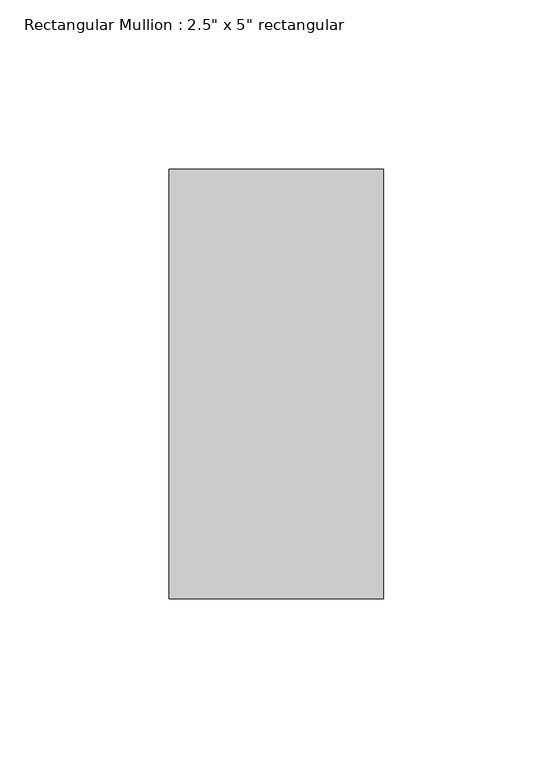
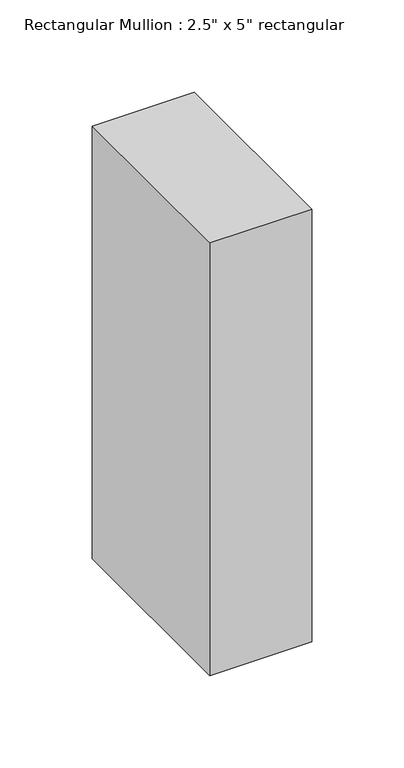
"""IFC4 building model written with IfcOpenShell, lengths in millimetres: member geometry."""

from ifc_helpers import new_model, si_unit, frame, origin, place, context, project, spatial, polyline, outline, extrude, source, transform, mapped, element, save


def member_6c34f49c(model_context):
    return source(origin(), model_context, "Body", "SweptSolid", [
        extrude(outline(polyline([(0.0, 63.5), (0.0, -63.5), (-63.5, -63.5), (-63.5, 63.5), (0.0, 63.5)])), frame((0.0, 0.0, -285.75), z_axis=(0.0, 0.0, 1.0), x_axis=(1.0, 0.0, 0.0)), (0.0, 0.0, 1.0), 285.75),
    ])


if __name__ == "__main__":
    model = new_model("IFC4")
    model_context = context("Model", 3, world=origin())
    ifc_project = project(units=[si_unit("LENGTHUNIT", "METRE", prefix="MILLI")], contexts=[model_context])
    site = spatial("IfcSite", under=ifc_project)
    building = spatial("IfcBuilding", under=site)
    placement = place(None, origin())
    member_shape = member_6c34f49c(model_context)
    element("IfcMember", 1, ObjectType="Rectangular Mullion : 2.5\" x 5\" rectangular", at=placement, inside=building, context=model_context, shape_type="MappedRepresentation", body=[
        mapped(member_shape, transform((0.0, 0.0, 0.0), x_axis=(1.0, 0.0, 0.0), y_axis=(0.0, 1.0, 0.0), z_axis=(0.0, 0.0, 1.0))),
    ])
    save(model, "model.ifc")

# Revit data of these elements
# Type "Rectangular Mullion : 2.5\" x 5\" rectangular"
#   built-in parameter 1007304 = 0.416667 (stored number, unit not read)
#   built-in parameter 1007301 = 0.104167 (stored number, unit not read)
#   built-in parameter 1007300 = 0.104167 (stored number, unit not read)
# Element 1 (IfcMember, "Rectangular Mullion : 2.5\" x 5\" rectangular")
#   Materials on its faces: "Aluminum"
# Materials
#   "Aluminum": class "Metal", colour RGB 247 247 247, transparency 0, Description = "Aluminum 6061", Cost = 0
